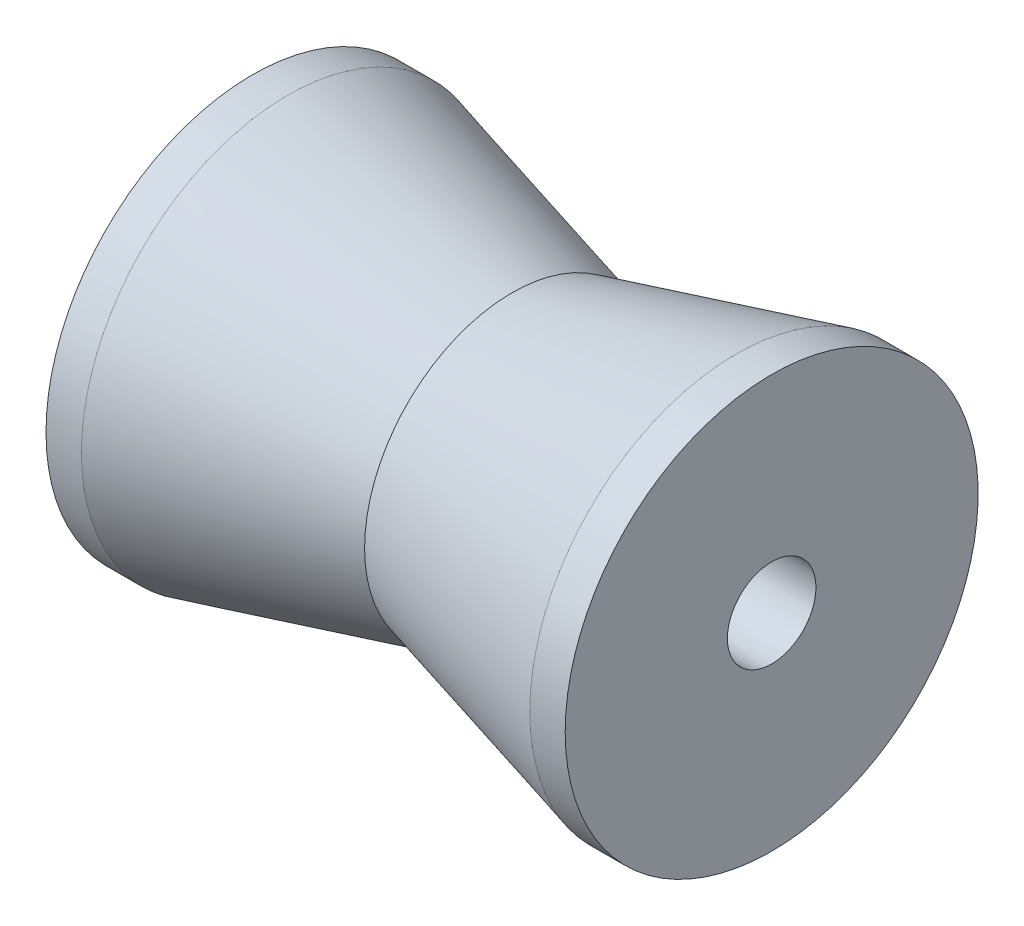
SolidWorks part; units mm, degrees
material "Plain Carbon Steel"
ref_plane "Front Plane" through (0, 0, 0) normal (0, 0, 1) x (1, 0, 0)
ref_plane "Top Plane" through (0, 0, 0) normal (0, 1, 0) x (1, 0, 0)
ref_plane "Right Plane" through (0, 0, 0) normal (1, 0, 0) x (0, 0, -1)
sketch "Roller Profile Sketch" plane through (0, 0, 0) normal (0, 0, 1) x (1, 0, 0)
  line L0 (0, 0) -> (0, 50) construction
  line L1 (0, 50) -> (-38, 60)
  line L2 (38, 60) -> (44, 60)
  line L4 (44, 60) -> (44, 32.5)
  line L5 (-38, 60) -> (-44, 60)
  line L8 (-44, 60) -> (-44, 32.5)
  line L11 (0, 50) -> (38, 60)
  line L12 (-44, 32.5) -> (44, 32.5)
  line L13 (-44, 25) -> (44, 25) construction
  point P8 (0, 25)
  dimension "D1" = 25
  dimension "D2" = 35
  dimension "D3" = 38
  dimension "D4" = 6
  dimension "D5" = 6
  dimension "D7" = 7.5
revolve "Roller Body Revolve" add sketch "Roller Profile Sketch" angle 360 about L13
